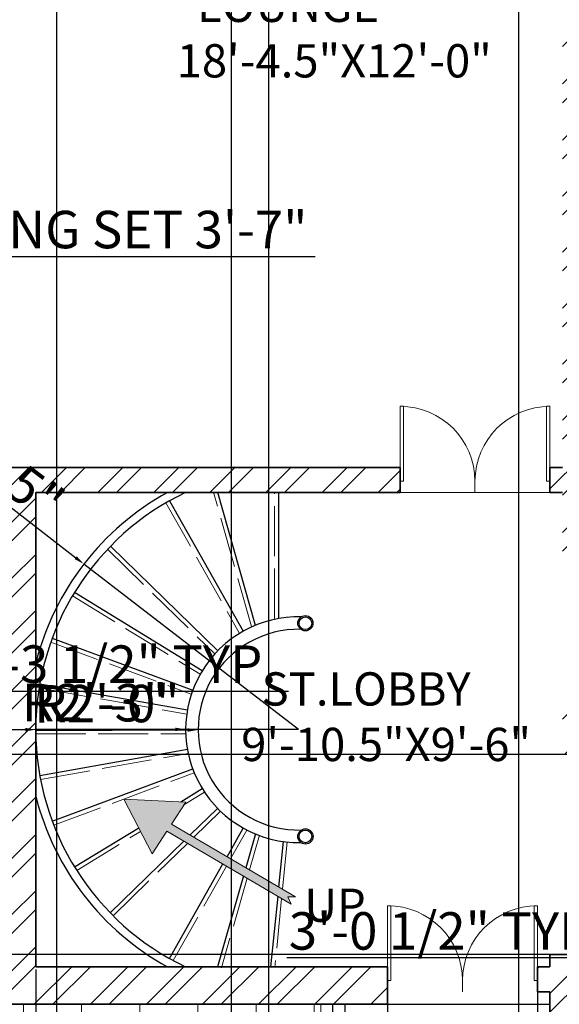
# Model space of a CAD drawing. Units: inches. Extents: x 287 to 905, y 1151 to 2037.
# Tile 3 of 5: x 516 to 646, y 1503 to 1739. Entities that reach past the tile are written whole.
import ezdxf

# ---------------------------------------------------------------- set-up
doc = ezdxf.new("R2010")
doc.units = ezdxf.units.IN
doc.linetypes.add('ACAD_ISO02W100', pattern=[15, 12, -3])
for name, color, linetype, lineweight in [('A-ANNO-DIMS', 2, 'Continuous', 18), ('A-ANNO-SYMB', 7, 'Continuous', 18), ('A-ANNO-TEXT', 7, 'Continuous', 25), ('A-AREA-IDEN', 7, 'Continuous', 18), ('A-DOOR', 4, 'Continuous', 18), ('A-FLOR-PATT', 252, 'Continuous', 13), ('A-FLOR-STRS', 7, 'Continuous', 25), ('A-FLOR-STRS-HIDN', 8, 'ACAD_ISO02W100', 13), ('A-WALL', 7, 'Continuous', 35), ('A-WALL-PATT', 252, 'Continuous', 13), ('L-PVMT', 8, 'Continuous', 18)]:
    doc.layers.add(name, color=color, linetype=linetype, lineweight=lineweight)
doc.layers.add('L-PLNT-PATT', color=116, linetype='Continuous', lineweight=13, true_color=0x136734)
doc.styles.get("Standard").update_dxf_attribs({"font": 'arial.ttf'})
doc.dimstyles.new('ISO-25', dxfattribs={"dimtxt": 9, "dimasz": 2.5, "dimexe": 1.25, "dimexo": 0.625, "dimtad": 1, "dimlunit": 3, "dimtxsty": 'Standard', "dimcen": 2.5, "dimadec": 0, "dimazin": 0, "dimtfac": 1, "dimtmove": 0, "dimatfit": 3, "dimfxl": 1, "dimarcsym": 0})

# ---------------------------------------------------------------- blocks, each defined once
blk = doc.blocks.new('*U2')
for p, q in [((0, 0), (0, -6)), ((40, 0), (40, -6))]:
    blk.add_line(p, q)
blk.add_lwpolyline([(0, 0), (0, 40), (1.75, 40), (1.75, 0)], close=True)
blk.add_arc((0, 0), 40, 0, 90)
blk = doc.blocks.new('*U3')
for p, q in [((0, 0), (0, -6)), ((-40, 0), (-40, -6))]:
    blk.add_line(p, q)
blk.add_lwpolyline([(0, 0), (0, 40), (-1.75, 40), (-1.75, 0)], close=True)
blk.add_arc((0, 0), 40, 90, 180)
blk = doc.blocks.new('*D25')
at = {"layer": 'A-ANNO-DIMS', "color": 0, "lineweight": -2, "transparency": 16777216}
for p, q in [((659.72, 1502.05), (659.72, 1515.27)), ((696.39, 1502.05), (696.39, 1515.27)), ((659.72, 1514.02), (580.15, 1514.02)), ((693.89, 1514.02), (662.22, 1514.02))]:
    blk.add_line(p, q, dxfattribs=at)
at = {"layer": 'A-ANNO-DIMS', "color": 0, "transparency": 16777216}
for points in [[(662.22, 1514.44), (662.22, 1513.61), (659.72, 1514.02)], [(693.89, 1514.44), (693.89, 1513.61), (696.39, 1514.02)]]:
    blk.add_solid(points, dxfattribs=at)
at = {"layer": 'Defpoints', "color": 0, "transparency": 16777216}
for p in [(659.72, 1514.02), (659.72, 1501.42), (696.39, 1501.42)]:
    blk.add_point(p, dxfattribs=at)
at = {"layer": 'A-ANNO-DIMS', "color": 0, "transparency": 16777216, "insert": (618.68, 1519.3), "char_height": 9, "attachment_point": 5}
blk.add_mtext('3\'-0 1/2" TYP.', dxfattribs=at)
blk = doc.blocks.new('*D26')
at = {"layer": 'A-ANNO-DIMS', "color": 0, "lineweight": -2, "transparency": 16777216}
for p, q in [((429.49, 1576.45), (429.49, 1579.37)), ((444.82, 1576.45), (444.82, 1579.37)), ((431.99, 1578.12), (442.32, 1578.12)), ((444.82, 1578.12), (580.58, 1578.12))]:
    blk.add_line(p, q, dxfattribs=at)
at = {"layer": 'A-ANNO-DIMS', "color": 0, "transparency": 16777216}
for points in [[(431.99, 1578.54), (431.99, 1577.71), (429.49, 1578.12)], [(442.32, 1578.54), (442.32, 1577.71), (444.82, 1578.12)]]:
    blk.add_solid(points, dxfattribs=at)
at = {"layer": 'Defpoints', "color": 0, "transparency": 16777216}
for p in [(429.49, 1575.83), (444.82, 1578.12), (444.82, 1575.83)]:
    blk.add_point(p, dxfattribs=at)
at = {"layer": 'A-ANNO-DIMS', "color": 0, "transparency": 16777216, "insert": (513.95, 1583.41), "char_height": 9, "attachment_point": 5}
blk.add_mtext('BURNER 1\'-3 1/2" TYP.', dxfattribs=at)
blk = doc.blocks.new('*D28')
at = {"layer": 'A-ANNO-DIMS', "color": 0, "lineweight": -2, "transparency": 16777216}
for p, q in [((441.2, 1676.71), (441.2, 1683.81)), ((443.7, 1682.56), (481.83, 1682.56)), ((484.33, 1676.71), (484.33, 1683.81)), ((484.33, 1682.56), (587, 1682.56))]:
    blk.add_line(p, q, dxfattribs=at)
at = {"layer": 'A-ANNO-DIMS', "color": 0, "transparency": 16777216}
for points in [[(443.7, 1682.97), (443.7, 1682.14), (441.2, 1682.56)], [(481.83, 1682.97), (481.83, 1682.14), (484.33, 1682.56)]]:
    blk.add_solid(points, dxfattribs=at)
at = {"layer": 'Defpoints', "color": 0, "transparency": 16777216}
for p in [(484.33, 1682.56), (441.2, 1676.09), (484.33, 1676.09)]:
    blk.add_point(p, dxfattribs=at)
at = {"layer": 'A-ANNO-DIMS', "color": 0, "transparency": 16777216, "insert": (536.92, 1687.84), "char_height": 9, "attachment_point": 5}
blk.add_mtext('DINING SET 3\'-7"', dxfattribs=at)
blk = doc.blocks.new('*D32')
at = {"layer": 'A-ANNO-DIMS', "color": 0, "lineweight": -2, "transparency": 16777216}
for p, q in [((426.39, 1284.46), (426.39, 2019.96)), ((428.89, 2018.71), (564.36, 2018.71)), ((566.86, 1284.46), (566.86, 2019.96))]:
    blk.add_line(p, q, dxfattribs=at)
at = {"layer": 'A-ANNO-DIMS', "color": 0, "transparency": 16777216}
for points in [[(428.89, 2019.12), (428.89, 2018.29), (426.39, 2018.71)], [(564.36, 2019.12), (564.36, 2018.29), (566.86, 2018.71)]]:
    blk.add_solid(points, dxfattribs=at)
at = {"layer": 'Defpoints', "color": 0, "transparency": 16777216}
for p in [(566.86, 2018.71), (426.39, 1283.83), (566.86, 1283.83)]:
    blk.add_point(p, dxfattribs=at)
at = {"layer": 'A-ANNO-DIMS', "color": 0, "transparency": 16777216, "insert": (496.62, 2023.99), "char_height": 9, "attachment_point": 5}
blk.add_mtext('11\'-8 1/2"', dxfattribs=at)
blk = doc.blocks.new('*D33')
at = {"layer": 'A-ANNO-DIMS', "color": 0, "lineweight": -2, "transparency": 16777216}
for p, q in [((575.86, 1284.46), (575.86, 2019.96)), ((578.36, 2018.71), (633.36, 2018.71)), ((635.86, 1284.46), (635.86, 2019.96))]:
    blk.add_line(p, q, dxfattribs=at)
at = {"layer": 'A-ANNO-DIMS', "color": 0, "transparency": 16777216}
for points in [[(578.36, 2019.12), (578.36, 2018.29), (575.86, 2018.71)], [(633.36, 2019.12), (633.36, 2018.29), (635.86, 2018.71)]]:
    blk.add_solid(points, dxfattribs=at)
at = {"layer": 'Defpoints', "color": 0, "transparency": 16777216}
for p in [(635.86, 2018.71), (575.86, 1283.83), (635.86, 1283.83)]:
    blk.add_point(p, dxfattribs=at)
at = {"layer": 'A-ANNO-DIMS', "color": 0, "transparency": 16777216, "insert": (605.86, 2023.93), "char_height": 9, "attachment_point": 5}
blk.add_mtext('5\'-0"', dxfattribs=at)
blk = doc.blocks.new('*D34')
at = {"layer": 'A-ANNO-DIMS', "color": 0, "lineweight": -2, "transparency": 16777216}
for p, q in [((604.36, 1511.21), (604.36, 1157.65)), ((640.36, 1511.21), (640.36, 1157.65)), ((606.86, 1158.9), (637.86, 1158.9))]:
    blk.add_line(p, q, dxfattribs=at)
at = {"layer": 'A-ANNO-DIMS', "color": 0, "transparency": 16777216}
for points in [[(606.86, 1159.32), (606.86, 1158.49), (604.36, 1158.9)], [(637.86, 1159.32), (637.86, 1158.49), (640.36, 1158.9)]]:
    blk.add_solid(points, dxfattribs=at)
at = {"layer": 'Defpoints', "color": 0, "transparency": 16777216}
for p in [(604.36, 1511.83), (640.36, 1511.83), (640.36, 1158.9)]:
    blk.add_point(p, dxfattribs=at)
at = {"layer": 'A-ANNO-DIMS', "color": 0, "transparency": 16777216, "insert": (622.36, 1164.13), "char_height": 9, "attachment_point": 5}
blk.add_mtext('3\'-0"', dxfattribs=at)
blk = doc.blocks.new('*D35')
at = {"layer": 'A-ANNO-DIMS', "color": 0, "lineweight": -2, "transparency": 16777216}
for p, q in [((651.73, 1562.83), (370.73, 1562.83)), ((371.98, 1517.33), (371.98, 1560.33)), ((651.73, 1514.83), (370.73, 1514.83))]:
    blk.add_line(p, q, dxfattribs=at)
at = {"layer": 'A-ANNO-DIMS', "color": 0, "transparency": 16777216}
for points in [[(371.57, 1560.33), (372.4, 1560.33), (371.98, 1562.83)], [(371.57, 1517.33), (372.4, 1517.33), (371.98, 1514.83)]]:
    blk.add_solid(points, dxfattribs=at)
at = {"layer": 'Defpoints', "color": 0, "transparency": 16777216}
for p in [(371.98, 1562.83), (652.36, 1562.83), (652.36, 1514.83)]:
    blk.add_point(p, dxfattribs=at)
at = {"layer": 'A-ANNO-DIMS', "color": 0, "transparency": 16777216, "insert": (366.76, 1538.83), "char_height": 9, "attachment_point": 5, "rotation": 90}
blk.add_mtext('4\'-0"', dxfattribs=at)
blk = doc.blocks.new('*D36')
at = {"layer": 'A-ANNO-DIMS', "color": 0, "lineweight": -2, "transparency": 16777216}
for p, q in [((513.86, 1511.21), (513.86, 1157.65)), ((519.86, 1511.21), (519.86, 1157.65)), ((511.36, 1158.9), (508.86, 1158.9)), ((513.86, 1158.9), (519.86, 1158.9)), ((522.36, 1158.9), (550.03, 1158.9))]:
    blk.add_line(p, q, dxfattribs=at)
at = {"layer": 'A-ANNO-DIMS', "color": 0, "transparency": 16777216}
for points in [[(511.36, 1159.32), (511.36, 1158.49), (513.86, 1158.9)], [(522.36, 1159.32), (522.36, 1158.49), (519.86, 1158.9)]]:
    blk.add_solid(points, dxfattribs=at)
at = {"layer": 'Defpoints', "color": 0, "transparency": 16777216}
for p in [(513.86, 1511.83), (519.86, 1511.83), (519.86, 1158.9)]:
    blk.add_point(p, dxfattribs=at)
at = {"layer": 'A-ANNO-DIMS', "color": 0, "transparency": 16777216, "insert": (537.44, 1164.12), "char_height": 9, "attachment_point": 5}
blk.add_mtext('0\'-6"', dxfattribs=at)
blk = doc.blocks.new('*D37')
at = {"layer": 'A-ANNO-DIMS', "color": 0, "lineweight": -2, "transparency": 16777216}
for p, q in [((524.86, 1967.21), (524.86, 1157.65)), ((686.86, 1967.21), (686.86, 1157.65)), ((527.36, 1158.9), (684.36, 1158.9))]:
    blk.add_line(p, q, dxfattribs=at)
at = {"layer": 'A-ANNO-DIMS', "color": 0, "transparency": 16777216}
for points in [[(527.36, 1159.32), (527.36, 1158.49), (524.86, 1158.9)], [(684.36, 1159.32), (684.36, 1158.49), (686.86, 1158.9)]]:
    blk.add_solid(points, dxfattribs=at)
at = {"layer": 'Defpoints', "color": 0, "transparency": 16777216}
for p in [(524.86, 1967.83), (686.86, 1967.83), (686.86, 1158.9)]:
    blk.add_point(p, dxfattribs=at)
at = {"layer": 'A-ANNO-DIMS', "color": 0, "transparency": 16777216, "insert": (605.86, 1164.13), "char_height": 9, "attachment_point": 5}
blk.add_mtext('13\'-6"', dxfattribs=at)
blk = doc.blocks.new('*D41')
at = {"layer": 'A-ANNO-DIMS', "color": 0, "lineweight": -2, "transparency": 16777216}
for p, q in [((479.4, 1648.76), (529.44, 1610.15)), ((582.98, 1568.83), (531.42, 1608.62))]:
    blk.add_line(p, q, dxfattribs=at)
at = {"layer": 'A-ANNO-DIMS', "color": 0, "transparency": 16777216}
blk.add_solid([(529.7, 1610.48), (529.19, 1609.82), (531.42, 1608.62)], dxfattribs=at)
at = {"layer": 'Defpoints', "color": 0, "transparency": 16777216}
for p in [(531.42, 1608.62), (582.98, 1568.83)]:
    blk.add_point(p, dxfattribs=at)
at = {"layer": 'A-ANNO-DIMS', "color": 0, "transparency": 16777216, "insert": (503.67, 1636.62), "char_height": 9, "attachment_point": 5, "rotation": 322.3456}
blk.add_mtext('2X R5\'-5"', dxfattribs=at)
blk = doc.blocks.new('*D42')
at = {"layer": 'A-ANNO-DIMS', "color": 0, "lineweight": -2, "transparency": 16777216}
for p, q in [((465.09, 1568.83), (517.36, 1568.83)), ((582.98, 1568.83), (519.86, 1568.83))]:
    blk.add_line(p, q, dxfattribs=at)
at = {"layer": 'A-ANNO-DIMS', "color": 0, "transparency": 16777216}
blk.add_solid([(517.36, 1569.25), (517.36, 1568.42), (519.86, 1568.83)], dxfattribs=at)
at = {"layer": 'Defpoints', "color": 0, "transparency": 16777216}
for p in [(519.86, 1568.83), (582.98, 1568.83)]:
    blk.add_point(p, dxfattribs=at)
at = {"layer": 'A-ANNO-DIMS', "color": 0, "transparency": 16777216, "insert": (481.98, 1574.06), "char_height": 9, "attachment_point": 5, "rotation": 0.0002}
blk.add_mtext('R5\'-3"', dxfattribs=at)
blk = doc.blocks.new('*D43')
at = {"layer": 'A-ANNO-DIMS', "color": 0, "lineweight": -2, "transparency": 16777216}
for p, q in [((517.07, 1568.97), (553.36, 1568.9)), ((582.98, 1568.83), (555.86, 1568.89))]:
    blk.add_line(p, q, dxfattribs=at)
at = {"layer": 'A-ANNO-DIMS', "color": 0, "transparency": 16777216}
blk.add_solid([(553.36, 1569.31), (553.36, 1568.48), (555.86, 1568.89)], dxfattribs=at)
at = {"layer": 'Defpoints', "color": 0, "transparency": 16777216}
for p in [(555.86, 1568.89), (582.98, 1568.83)]:
    blk.add_point(p, dxfattribs=at)
at = {"layer": 'A-ANNO-DIMS', "color": 0, "transparency": 16777216, "insert": (533.97, 1574.16), "char_height": 9, "attachment_point": 5, "rotation": 359.8781}
blk.add_mtext('R2\'-3"', dxfattribs=at)
blk = doc.blocks.new('*D44')
at = {"layer": 'A-ANNO-DIMS', "color": 0, "lineweight": -2, "transparency": 16777216}
for p, q in [((520.07, 1568.66), (556.36, 1568.76)), ((582.98, 1568.83), (558.86, 1568.77))]:
    blk.add_line(p, q, dxfattribs=at)
at = {"layer": 'A-ANNO-DIMS', "color": 0, "transparency": 16777216}
blk.add_solid([(556.36, 1569.17), (556.36, 1568.34), (558.86, 1568.77)], dxfattribs=at)
at = {"layer": 'Defpoints', "color": 0, "transparency": 16777216}
for p in [(558.86, 1568.77), (582.98, 1568.83)]:
    blk.add_point(p, dxfattribs=at)
at = {"layer": 'A-ANNO-DIMS', "color": 0, "transparency": 16777216, "insert": (536.95, 1573.92), "char_height": 9, "attachment_point": 5, "rotation": 0.1621}
blk.add_mtext('R2\'-0"', dxfattribs=at)

msp = doc.modelspace()

# ---------------------------------------------------------------- hatches: boundary and pattern name
at = {"layer": 'A-ANNO-SYMB'}
h = msp.add_hatch(color=256, dxfattribs=at)
h.dxf.hatch_style = 1
h.paths.add_polyline_path([(555.86, 1551.444), (541.035, 1552.169), (547.82, 1538.967), (551.37, 1544.476), (581.237, 1526.899), (580.376, 1528.622), (582.251, 1528.622), (552.454, 1546.159)])
at = {"layer": 'A-FLOR-PATT'}
h = msp.add_hatch(dxfattribs=at)
h.set_pattern_fill('ANGLE', color=256, scale=2)
h.set_pattern_definition([(0, (0, 0), (0, 13.97), [10.16, -3.81]), (90, (0, 0), (-13.97, 9e-16), [10.16, -3.81])])
h.paths.add_polyline_path([(588.313, 1502.833), (422.857, 1502.833), (422.857, 1283.833), (588.313, 1283.833)])
h.paths.add_polyline_path([(486.188, 1389.005), (563.901, 1389.005), (563.901, 1418.856), (486.188, 1418.856)], flags=24)
at = {"layer": 'A-WALL-PATT'}
h = msp.add_hatch(dxfattribs=at)
h.set_pattern_fill('ANSI32', color=256)
h.paths.add_polyline_path([(604.357, 1511.833), (519.857, 1511.833), (519.857, 1625.833), (607.357, 1625.833), (607.357, 1631.833), (510.857, 1631.833), (510.857, 1625.833), (513.857, 1625.833), (513.857, 1511.833), (496.063, 1511.833), (496.063, 1502.833), (604.357, 1502.833)])
h.paths.add_polyline_path([(652.357, 1511.833), (652.357, 1514.833), (643.357, 1514.833), (643.357, 1511.833), (640.357, 1511.833), (640.357, 1505.833), (643.357, 1505.833), (643.357, 1370.833), (690.607, 1370.833), (690.607, 1379.833), (652.357, 1379.833)])
h.paths.add_polyline_path([(797.857, 1582.055), (788.857, 1582.055), (788.857, 1571.833), (703.357, 1571.833), (703.357, 1574.833), (697.357, 1574.833), (697.357, 1571.833), (652.357, 1571.833), (652.357, 1574.833), (646.357, 1574.833), (646.357, 1562.833), (652.357, 1562.833), (652.357, 1565.833), (788.857, 1565.833), (788.857, 1379.833), (750.607, 1379.833), (750.607, 1370.833), (797.857, 1370.833)])
h.paths.add_polyline_path([(797.857, 1673.833), (788.857, 1673.833), (788.857, 1631.833), (685.357, 1631.833), (685.357, 1625.833), (697.357, 1625.833), (697.357, 1604.833), (703.357, 1604.833), (703.357, 1625.833), (788.857, 1625.833), (788.857, 1603.055), (797.857, 1603.055)])
h.paths.add_polyline_path([(797.857, 1976.833), (751.357, 1976.833), (751.357, 1967.833), (788.857, 1967.833), (788.857, 1919.833), (785.857, 1919.833), (785.857, 1913.833), (788.857, 1913.833), (788.857, 1781.833), (654.342, 1781.833), (643.328, 1792.848), (639.085, 1788.605), (645.857, 1781.833), (645.857, 1775.833), (646.357, 1775.833), (646.357, 1772.833), (652.357, 1772.833), (652.357, 1775.833), (788.857, 1775.833), (788.857, 1733.833), (797.857, 1733.833)])
h.paths.add_polyline_path([(755.857, 1919.833), (692.857, 1919.833), (692.857, 1967.833), (730.357, 1967.833), (730.357, 1976.833), (473.78, 1976.833), (473.78, 1967.833), (518.857, 1967.833), (518.857, 1919.833), (455.857, 1919.833), (455.857, 1913.833), (567.857, 1913.833), (567.857, 1919.833), (524.857, 1919.833), (524.857, 1967.833), (686.857, 1967.833), (686.857, 1919.833), (639.857, 1919.833), (639.857, 1913.833), (755.857, 1913.833)])
h.paths.add_polyline_path([(606.857, 1913.833), (609.857, 1913.833), (609.857, 1919.833), (597.857, 1919.833), (597.857, 1913.833), (600.857, 1913.833), (600.857, 1829.319), (589.842, 1818.304), (594.085, 1814.061), (600.857, 1820.833), (600.857, 1781.833), (597.857, 1781.833), (597.857, 1775.833), (609.857, 1775.833), (609.857, 1781.833), (606.857, 1781.833), (606.857, 1820.833), (613.629, 1814.061), (617.872, 1818.304), (606.857, 1829.319)])
h.paths.add_polyline_path([(652.357, 1736.833), (646.357, 1736.833), (646.357, 1631.833), (643.357, 1631.833), (643.357, 1625.833), (646.357, 1625.833), (646.357, 1604.833), (652.357, 1604.833), (652.357, 1625.833), (655.357, 1625.833), (655.357, 1631.833), (652.357, 1631.833)])
at = {"layer": 'L-PLNT-PATT'}
h = msp.add_hatch(dxfattribs=at)
h.set_pattern_fill('CROSS', color=256, scale=2)
h.paths.add_polyline_path([(788.857, 1283.833), (788.857, 1370.833), (643.357, 1370.833), (643.357, 1477.833), (594.127, 1477.833), (594.127, 1475.527, -0.1568242), (594.486, 1474.41, -1), (590.655, 1474.41, -0.1814073), (591.127, 1475.671), (591.127, 1502.833), (588.313, 1502.833), (588.313, 1283.833)])
h.paths.add_polyline_path([(640.902, 1304.954), (590.891, 1304.954), (590.891, 1328.274), (640.902, 1328.274)], flags=16)
h.paths.add_polyline_path([(638.902, 1306.954), (592.891, 1306.954), (592.891, 1326.274), (638.902, 1326.274)], flags=0)
h.paths.add_polyline_path([(640.902, 1340.02), (590.891, 1340.02), (590.891, 1363.34), (640.902, 1363.34)], flags=16)
h.paths.add_polyline_path([(638.902, 1342.02), (592.891, 1342.02), (592.891, 1361.34), (638.902, 1361.34)], flags=0)
h.paths.add_polyline_path([(640.902, 1371.662), (590.891, 1371.662), (590.891, 1394.982), (640.902, 1394.982)], flags=16)
h.paths.add_polyline_path([(638.902, 1373.662), (592.891, 1373.662), (592.891, 1392.982), (638.902, 1392.982)], flags=0)
h.paths.add_polyline_path([(640.902, 1406.128), (590.891, 1406.128), (590.891, 1429.448), (640.902, 1429.448)], flags=16)
h.paths.add_polyline_path([(638.902, 1408.128), (592.891, 1408.128), (592.891, 1427.448), (638.902, 1427.448)], flags=0)
h.paths.add_polyline_path([(640.902, 1439.308), (590.891, 1439.308), (590.891, 1462.628), (640.902, 1462.628)], flags=16)
h.paths.add_polyline_path([(638.902, 1441.308), (592.891, 1441.308), (592.891, 1460.628), (638.902, 1460.628)], flags=0)
h.paths.add_polyline_path([(678.527, 1323.107), (756.41, 1323.107), (756.41, 1352.959), (678.527, 1352.959)], flags=24)

# ---------------------------------------------------------------- linework, layer by layer
at = {"layer": 'A-ANNO-SYMB'}
for p, q in [((582.251, 1528.622), (552.454, 1546.159)), ((581.237, 1526.899), (551.37, 1544.476)), ((582.251, 1528.622), (580.376, 1528.622)), ((580.376, 1528.622), (581.237, 1526.899))]:
    msp.add_line(p, q, dxfattribs=at)
msp.add_lwpolyline([(552.454, 1546.159), (555.86, 1551.444), (541.035, 1552.169), (547.82, 1538.967), (551.37, 1544.476)], dxfattribs=at)
at = {"layer": 'A-DOOR'}
msp.add_line((607.357, 1625.833), (643.357, 1625.833), dxfattribs=at)
at = {"layer": 'A-FLOR-STRS'}
for p, q in [((572.616, 1593.899), (563.607, 1625.833)), ((578.216, 1595.536), (578.216, 1625.833)), ((552.002, 1623.833), (569.67, 1592.467)), ((537.857, 1612.833), (563.561, 1587.77)), ((529.17, 1601.833), (559.859, 1583.013)), ((523.815, 1590.833), (557.558, 1578.287)), ((520.823, 1579.833), (556.272, 1573.56)), ((519.857, 1568.833), (555.857, 1568.833)), ((520.823, 1557.833), (556.272, 1564.107)), ((523.815, 1546.833), (557.558, 1559.38)), ((554.717, 1551.5), (559.859, 1554.653)), ((556.941, 1543.519), (563.532, 1549.926)), ((529.17, 1535.833), (544.575, 1545.28)), ((565.79, 1538.311), (569.67, 1545.2)), ((572.616, 1543.767), (570.3, 1535.656)), ((537.719, 1524.833), (555.454, 1542.073)), ((579.264, 1541.964), (578.176, 1531.021)), ((552.002, 1513.833), (564.808, 1536.568)), ((569.733, 1533.669), (563.501, 1511.833)), ((577.958, 1528.829), (576.268, 1511.833)), ((591.127, 1502.833), (591.127, 1475.671)), ((594.127, 1502.833), (594.127, 1475.527)), ((604.357, 1502.833), (643.357, 1502.833))]:
    msp.add_line(p, q, dxfattribs=at)
for centre, radius in [((584.616, 1594.406), 1.828), ((584.616, 1594.406), 1.528), ((584.622, 1543.173), 1.828), ((584.622, 1543.173), 1.528)]:
    msp.add_circle(centre, radius, dxfattribs=at)
for radius, start, end in [(63.125, 115.44871, 244.55129), (65.125, 118.92662, 165.76372), (27.125, 88.61367, 271.14087), (24.125, 88.75179, 271.57467), (65.125, 194.23628, 241.07338)]:
    msp.add_arc((582.982, 1568.833), radius, start, end, dxfattribs=at)
at = {"layer": 'A-FLOR-STRS-HIDN'}
for p, q in [((571.653, 1593.628), (562.645, 1625.562)), ((577.216, 1595.536), (577.216, 1625.833)), ((551.131, 1623.342), (568.799, 1591.976)), ((537.159, 1612.117), (562.863, 1587.054)), ((528.647, 1600.981), (559.336, 1582.161)), ((523.466, 1589.896), (557.209, 1577.349)), ((520.649, 1578.849), (556.098, 1572.575)), ((519.857, 1567.833), (555.857, 1567.833)), ((520.997, 1556.849), (556.446, 1563.122)), ((524.163, 1545.896), (557.906, 1558.443)), ((555.417, 1550.756), (560.382, 1553.801)), ((557.834, 1542.993), (564.229, 1549.209)), ((529.693, 1534.981), (545.034, 1544.389)), ((566.652, 1537.803), (570.541, 1544.709)), ((573.577, 1543.493), (571.191, 1535.132)), ((538.416, 1524.116), (556.347, 1541.547)), ((580.259, 1541.865), (579.125, 1530.462)), ((552.873, 1513.342), (565.67, 1536.06)), ((570.624, 1533.145), (564.462, 1511.559)), ((578.907, 1528.27), (577.263, 1511.734))]:
    msp.add_line(p, q, dxfattribs=at)
at = {"layer": 'A-WALL'}
for p, q in [((510.857, 1631.833), (607.357, 1631.833)), ((607.357, 1625.833), (607.357, 1631.833)), ((643.357, 1625.833), (643.357, 1631.833)), ((643.357, 1631.833), (646.357, 1631.833)), ((519.857, 1625.833), (519.857, 1511.833)), ((519.857, 1625.833), (607.357, 1625.833)), ((643.357, 1625.833), (646.357, 1625.833)), ((643.357, 1514.833), (652.357, 1514.833)), ((643.357, 1511.833), (643.357, 1514.833)), ((519.857, 1511.833), (604.357, 1511.833)), ((604.357, 1502.833), (604.357, 1511.833)), ((640.357, 1505.833), (640.357, 1511.833)), ((640.357, 1511.833), (643.357, 1511.833)), ((640.357, 1505.833), (643.357, 1505.833)), ((643.357, 1505.833), (643.357, 1370.833)), ((413.857, 1502.833), (604.357, 1502.833))]:
    msp.add_line(p, q, dxfattribs=at)
at = {"layer": 'L-PVMT'}
msp.add_line((588.313, 1283.833), (588.313, 1502.833), dxfattribs=at)

# ---------------------------------------------------------------- block references
at = {"layer": 'A-DOOR', "xscale": 0.45, "yscale": 0.45, "zscale": 0.45}
for name, p in [('*U2', (607.357, 1628.533)), ('*U3', (643.357, 1628.533)), ('*U2', (604.357, 1508.533)), ('*U3', (640.357, 1508.533))]:
    msp.add_blockref(name, p, dxfattribs=at)

# ---------------------------------------------------------------- texts
at = {"layer": 'A-ANNO-TEXT', "insert": (584.352, 1530.631), "char_height": 8, "attachment_point": 1}
msp.add_mtext_dynamic_manual_height_columns('UP', width=16.25186, gutter_width=12.5, heights=[0], dxfattribs=at)
at = {"layer": 'A-AREA-IDEN', "char_height": 8, "attachment_point": 1}
for s, width, insert in [('  LOUNGE\\P18\'-4.5"X12\'-0"', 72.39263, (553.702, 1746.891)), ('  ST.LOBBY\\P9\'-10.5"X9\'-6"', 67.07303, (569.195, 1582.615))]:
    msp.add_mtext_dynamic_manual_height_columns(s, width=width, gutter_width=12.5, heights=[0], dxfattribs=dict(at, insert=insert))

# ---------------------------------------------------------------- dimensions: what is measured, and where the dimension line sits
at = {"layer": 'A-ANNO-DIMS'}
for base, p1, p2, picture, middle in [((566.857, 2018.708), (426.388, 1283.833), (566.857, 1283.833), '*D32', (496.622, 2023.987)), ((635.857, 2018.708), (575.857, 1283.833), (635.857, 1283.833), '*D33', (605.857, 2023.928)), ((686.857, 1158.902), (524.857, 1967.833), (686.857, 1967.833), '*D37', (605.857, 1164.125)), ((519.857, 1158.902), (513.857, 1511.833), (519.857, 1511.833), '*D36', (537.444, 1164.122)), ((640.357, 1158.902), (604.357, 1511.833), (640.357, 1511.833), '*D34', (622.357, 1164.125))]:
    dim = msp.add_linear_dim(base=base, p1=p1, p2=p2, dimstyle='ISO-25', override={"dimdec": 1, "dimlfac": 1, "dimrnd": 0, "dimzin": 1, "dimdsep": 46, "dimlunit": 4, "dimfrac": 2}, dxfattribs=at)
    dim.commit()
    dim.dimension.update_dxf_attribs({"geometry": picture, "text_midpoint": middle})
for base, p1, p2, text, picture, middle in [((484.333, 1682.557), (441.204, 1676.088), (484.333, 1676.088), 'DINING SET <>', '*D28', (536.918, 1687.839)), ((444.817, 1578.125), (429.487, 1575.825), (444.817, 1575.825), 'BURNER <> TYP.', '*D26', (513.95, 1583.406))]:
    dim = msp.add_linear_dim(base=base, p1=p1, p2=p2, text=text, dimstyle='ISO-25', override={"dimdec": 1, "dimlfac": 1, "dimrnd": 0, "dimzin": 1, "dimdsep": 46, "dimlunit": 4, "dimfrac": 2}, dxfattribs=at)
    dim.commit()
    dim.dimension.update_dxf_attribs({"geometry": picture, "text_midpoint": middle})
dim = msp.add_radius_dim(center=(582.982, 1568.833), mpoint=(531.422, 1608.618), text='2X <>', dimstyle='ISO-25', override={"dimdec": 1, "dimlfac": 1, "dimrnd": 0, "dimzin": 1, "dimdsep": 46, "dimlunit": 4, "dimfrac": 2}, dxfattribs=at)
dim.commit()
dim.dimension.update_dxf_attribs({"geometry": '*D41', "text_midpoint": (500.486, 1632.489), "dimtype": 164})
dim = msp.add_radius_dim(center=(582.982, 1568.833), mpoint=(519.857, 1568.833), dimstyle='ISO-25', override={"dimdec": 1, "dimlfac": 1, "dimrnd": 0, "dimzin": 1, "dimdsep": 46, "dimlunit": 4, "dimfrac": 2}, dxfattribs=at)
dim.commit()
dim.dimension.update_dxf_attribs({"geometry": '*D42', "text_midpoint": (481.982, 1568.833), "dimtype": 164})
for mpoint, picture, middle in [((555.857, 1568.891), '*D43', (533.975, 1574.161)), ((558.857, 1568.765), '*D44', (536.949, 1573.923))]:
    dim = msp.add_radius_dim(center=(582.982, 1568.833), mpoint=mpoint, dimstyle='ISO-25', override={"dimdec": 1, "dimlfac": 1, "dimrnd": 0, "dimzin": 1, "dimdsep": 46, "dimlunit": 4, "dimfrac": 2}, dxfattribs=at)
    dim.commit()
    dim.dimension.update_dxf_attribs({"geometry": picture, "text_midpoint": middle})
dim = msp.add_linear_dim(base=(371.982, 1562.833), p1=(652.357, 1514.833), p2=(652.357, 1562.833), angle=90, dimstyle='ISO-25', override={"dimdec": 1, "dimlfac": 1, "dimrnd": 0, "dimzin": 1, "dimdsep": 46, "dimlunit": 4, "dimfrac": 2}, dxfattribs=at)
dim.commit()
dim.dimension.update_dxf_attribs({"geometry": '*D35', "text_midpoint": (366.762, 1538.833)})
dim = msp.add_linear_dim(base=(659.721, 1514.022), p1=(696.388, 1501.422), p2=(659.721, 1501.422), angle=180, text='<> TYP.', dimstyle='ISO-25', override={"dimdec": 1, "dimlfac": 1, "dimrnd": 0, "dimzin": 1, "dimdsep": 46, "dimlunit": 4, "dimfrac": 2}, dxfattribs=at)
dim.commit()
dim.dimension.update_dxf_attribs({"geometry": '*D25', "text_midpoint": (618.684, 1519.304)})

doc.saveas('drawing.dxf')
